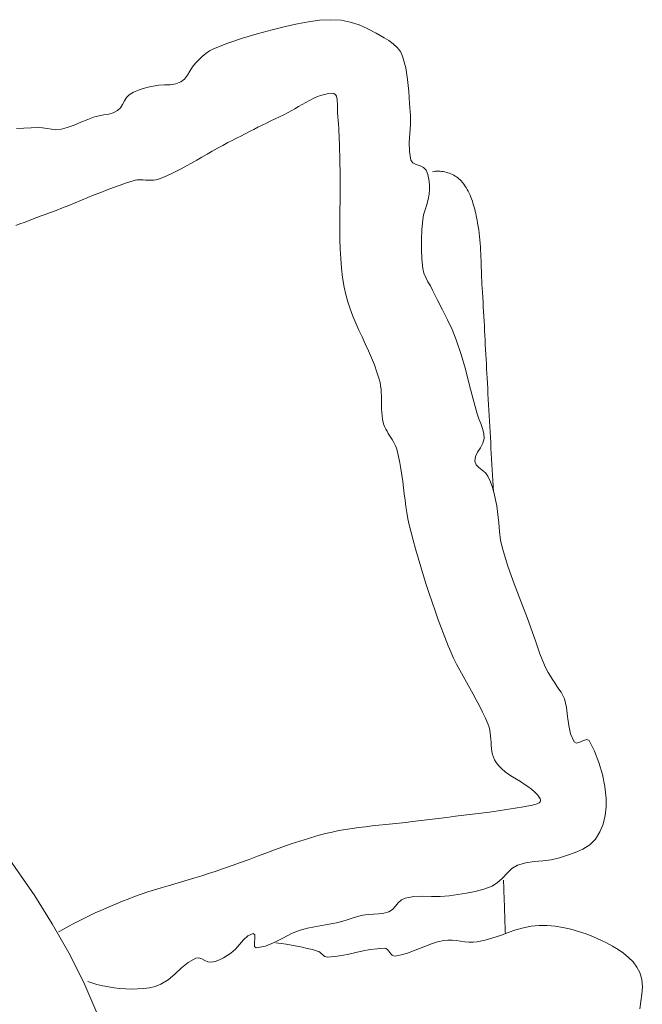
# Model space of a CAD drawing. Units: inches. Extents: x -36302355 to 648, y -221479757 to 75.
# Tile 20 of 37: x 572 to 589, y -501 to -475. Entities that reach past the tile are written whole.
import ezdxf

# ---------------------------------------------------------------- set-up
doc = ezdxf.new("R2010")
doc.units = ezdxf.units.IN
doc.header["$MEASUREMENT"] = 0
doc.layers.add('A-FURN', color=8, linetype='Continuous', lineweight=13)

# ---------------------------------------------------------------- blocks, each defined once
blk = doc.blocks.new('BED-DOUBLE')
for p, q in [((26.757, 79.348), (26.607, 79.27)), ((26.943, 79.401), (26.757, 79.348)), ((27.135, 79.418), (26.943, 79.401)), ((27.332, 79.407), (27.135, 79.418)), ((27.532, 79.381), (27.332, 79.407)), ((27.733, 79.348), (27.532, 79.381)), ((26.347, 79.049), (26.235, 78.914)), ((26.471, 79.169), (26.347, 79.049)), ((26.607, 79.27), (26.471, 79.169)), ((26.235, 78.914), (26.134, 78.768)), ((26.042, 78.615), (25.959, 78.459)), ((26.134, 78.768), (26.042, 78.615)), ((20.815, 78.133), (21.12, 78.252)), ((21.12, 78.252), (21.435, 78.344)), ((21.435, 78.344), (21.756, 78.407)), ((21.756, 78.407), (22.08, 78.443)), ((22.08, 78.443), (22.309, 78.445)), ((22.309, 78.445), (22.541, 78.42)), ((22.541, 78.42), (22.768, 78.366)), ((22.768, 78.366), (22.981, 78.28)), ((22.981, 78.28), (23.172, 78.159)), ((25.883, 78.303), (25.797, 78.108)), ((25.959, 78.459), (25.883, 78.303)), ((20.495, 77.926), (20.524, 77.986)), ((20.524, 77.986), (20.815, 78.133)), ((23.172, 78.159), (23.323, 78.006)), ((23.323, 78.006), (23.44, 77.822)), ((25.797, 78.108), (25.719, 77.908)), ((20.521, 77.836), (20.495, 77.926)), ((20.567, 77.736), (20.521, 77.836)), ((20.594, 77.646), (20.567, 77.736)), ((23.44, 77.822), (23.532, 77.618)), ((25.719, 77.908), (25.65, 77.704)), ((20.119, 77.44), (20.35, 77.491)), ((20.35, 77.491), (20.565, 77.584)), ((20.565, 77.584), (20.594, 77.646)), ((23.532, 77.618), (23.607, 77.405)), ((25.593, 77.496), (25.546, 77.286)), ((25.65, 77.704), (25.593, 77.496)), ((19.147, 77.177), (19.23, 77.234)), ((19.23, 77.234), (19.317, 77.284)), ((19.317, 77.284), (19.408, 77.323)), ((19.408, 77.323), (19.64, 77.378)), ((19.64, 77.378), (19.88, 77.41)), ((19.88, 77.41), (20.119, 77.44)), ((23.607, 77.405), (23.677, 77.194)), ((23.677, 77.194), (23.73, 76.972)), ((25.546, 77.286), (25.513, 77.074)), ((18.7, 76.891), (18.794, 76.949)), ((18.794, 76.949), (18.887, 77.007)), ((18.887, 77.007), (18.98, 77.065)), ((18.98, 77.065), (19.065, 77.119)), ((19.065, 77.119), (19.147, 77.177)), ((23.73, 76.972), (23.756, 76.743)), ((25.513, 77.074), (25.494, 76.862)), ((18.038, 76.614), (18.196, 76.668)), ((18.196, 76.668), (18.352, 76.726)), ((18.352, 76.726), (18.506, 76.789)), ((18.506, 76.789), (18.605, 76.837)), ((18.605, 76.837), (18.7, 76.891)), ((21.997, 76.607), (22.092, 76.675)), ((22.092, 76.675), (22.122, 76.687)), ((22.122, 76.687), (22.15, 76.685)), ((22.15, 76.685), (22.174, 76.67)), ((22.174, 76.67), (22.196, 76.645)), ((23.756, 76.743), (23.776, 76.512)), ((25.494, 76.862), (25.489, 76.649)), ((17.253, 76.332), (17.722, 76.507)), ((17.722, 76.507), (17.88, 76.561)), ((17.88, 76.561), (18.038, 76.614)), ((21.761, 76.345), (21.833, 76.44)), ((21.833, 76.44), (21.911, 76.527)), ((21.911, 76.527), (21.997, 76.607)), ((22.196, 76.645), (22.215, 76.61)), ((22.215, 76.61), (22.232, 76.569)), ((22.232, 76.569), (22.247, 76.522)), ((22.247, 76.522), (22.26, 76.472)), ((22.26, 76.472), (22.271, 76.419)), ((22.271, 76.419), (22.281, 76.367)), ((23.776, 76.512), (23.809, 76.285)), ((25.489, 76.649), (25.507, 76.436)), ((25.507, 76.436), (25.55, 76.227)), ((16.318, 75.975), (16.786, 76.152)), ((16.786, 76.152), (17.253, 76.332)), ((21.565, 76.038), (21.628, 76.142)), ((21.628, 76.142), (21.693, 76.245)), ((21.693, 76.245), (21.761, 76.345)), ((22.281, 76.367), (22.29, 76.317)), ((22.29, 76.317), (22.297, 76.271)), ((22.297, 76.271), (22.304, 76.23)), ((22.304, 76.23), (22.343, 76.002)), ((23.809, 76.285), (23.875, 76.067)), ((25.55, 76.227), (25.61, 76.02)), ((15.847, 75.807), (16.318, 75.975)), ((21.434, 75.833), (21.5, 75.934)), ((21.5, 75.934), (21.565, 76.038)), ((22.343, 76.002), (22.38, 75.774)), ((23.875, 76.067), (23.965, 75.917)), ((23.965, 75.917), (24.086, 75.786)), ((25.61, 76.02), (25.681, 75.814)), ((14.916, 75.581), (15.145, 75.609)), ((15.145, 75.609), (15.37, 75.658)), ((15.37, 75.658), (15.847, 75.807)), ((21.205, 75.561), (21.288, 75.644)), ((21.288, 75.644), (21.364, 75.736)), ((21.364, 75.736), (21.434, 75.833)), ((22.38, 75.774), (22.414, 75.545)), ((24.086, 75.786), (24.218, 75.662)), ((24.218, 75.662), (24.341, 75.531)), ((24.272, 75.689), (24.344, 75.691)), ((24.344, 75.691), (24.416, 75.694)), ((24.416, 75.694), (24.488, 75.697)), ((24.488, 75.697), (24.56, 75.699)), ((24.56, 75.699), (24.632, 75.702)), ((24.632, 75.702), (24.704, 75.704)), ((24.704, 75.704), (24.776, 75.707)), ((24.776, 75.707), (24.848, 75.709)), ((24.848, 75.709), (24.92, 75.712)), ((24.92, 75.712), (24.992, 75.714)), ((24.992, 75.714), (25.064, 75.717)), ((25.064, 75.717), (25.136, 75.719)), ((25.136, 75.719), (25.208, 75.722)), ((25.208, 75.722), (25.28, 75.724)), ((25.28, 75.724), (25.353, 75.727)), ((25.353, 75.727), (25.425, 75.729)), ((25.425, 75.729), (25.497, 75.732)), ((25.497, 75.732), (25.569, 75.734)), ((25.569, 75.734), (25.641, 75.737)), ((25.641, 75.737), (25.713, 75.74)), ((25.681, 75.814), (25.756, 75.609)), ((25.756, 75.609), (25.827, 75.404)), ((12.238, 75.329), (12.384, 75.337)), ((12.384, 75.337), (12.53, 75.345)), ((12.53, 75.345), (12.675, 75.353)), ((12.675, 75.353), (12.821, 75.362)), ((12.821, 75.362), (12.966, 75.37)), ((12.966, 75.37), (13.112, 75.378)), ((13.112, 75.378), (13.258, 75.386)), ((13.258, 75.386), (13.403, 75.395)), ((13.403, 75.395), (13.549, 75.403)), ((13.425, 75.27), (13.578, 75.336)), ((13.549, 75.403), (13.694, 75.411)), ((13.578, 75.336), (13.736, 75.39)), ((13.694, 75.411), (13.84, 75.419)), ((13.736, 75.39), (13.898, 75.435)), ((13.898, 75.435), (14.062, 75.473)), ((14.062, 75.473), (14.226, 75.506)), ((14.226, 75.506), (14.454, 75.541)), ((14.454, 75.541), (14.685, 75.562)), ((14.685, 75.562), (14.916, 75.581)), ((20.248, 75.322), (20.328, 75.335)), ((20.328, 75.335), (20.41, 75.344)), ((20.41, 75.344), (20.493, 75.35)), ((20.493, 75.35), (20.576, 75.355)), ((20.576, 75.355), (20.658, 75.36)), ((20.658, 75.36), (20.74, 75.367)), ((20.74, 75.367), (20.82, 75.378)), ((20.82, 75.378), (20.898, 75.394)), ((20.898, 75.394), (20.973, 75.417)), ((20.973, 75.417), (21.045, 75.447)), ((21.045, 75.447), (21.112, 75.488)), ((21.112, 75.488), (21.205, 75.561)), ((22.414, 75.545), (22.446, 75.315)), ((24.341, 75.531), (24.434, 75.383)), ((24.434, 75.383), (24.518, 75.161)), ((25.827, 75.404), (25.889, 75.196)), ((7.272, 75.067), (7.363, 75.072)), ((7.363, 75.072), (7.455, 75.077)), ((7.455, 75.077), (7.547, 75.081)), ((7.547, 75.081), (7.639, 75.085)), ((7.639, 75.085), (7.73, 75.088)), ((7.73, 75.088), (7.822, 75.091)), ((7.822, 75.091), (7.914, 75.095)), ((7.914, 75.095), (8.006, 75.098)), ((8.006, 75.098), (8.098, 75.102)), ((8.098, 75.102), (8.189, 75.106)), ((8.189, 75.106), (8.281, 75.11)), ((8.281, 75.11), (8.372, 75.116)), ((8.372, 75.116), (8.5, 75.124)), ((8.5, 75.124), (8.628, 75.131)), ((8.628, 75.131), (8.756, 75.139)), ((8.756, 75.139), (8.883, 75.146)), ((8.883, 75.146), (9.011, 75.154)), ((9.011, 75.154), (9.139, 75.161)), ((9.139, 75.161), (9.267, 75.168)), ((9.267, 75.168), (9.394, 75.175)), ((9.394, 75.175), (9.522, 75.181)), ((9.522, 75.181), (9.65, 75.188)), ((9.65, 75.188), (9.778, 75.195)), ((9.778, 75.195), (9.906, 75.201)), ((9.906, 75.201), (10.033, 75.208)), ((10.033, 75.208), (10.161, 75.215)), ((10.161, 75.215), (10.289, 75.221)), ((10.289, 75.221), (10.417, 75.228)), ((10.417, 75.228), (10.545, 75.235)), ((10.545, 75.235), (10.672, 75.242)), ((10.672, 75.242), (10.8, 75.248)), ((10.8, 75.248), (10.928, 75.255)), ((10.928, 75.255), (11.074, 75.264)), ((11.074, 75.264), (11.219, 75.272)), ((11.219, 75.272), (11.365, 75.28)), ((11.365, 75.28), (11.511, 75.288)), ((11.511, 75.288), (11.656, 75.296)), ((11.656, 75.296), (11.802, 75.304)), ((11.802, 75.304), (11.947, 75.312)), ((11.888, 75.025), (12.019, 75.077)), ((11.947, 75.312), (12.093, 75.321)), ((12.019, 75.077), (12.151, 75.125)), ((12.093, 75.321), (12.238, 75.329)), ((12.151, 75.125), (12.284, 75.159)), ((12.284, 75.159), (12.419, 75.168)), ((12.419, 75.168), (12.546, 75.136)), ((12.546, 75.136), (12.666, 75.069)), ((12.666, 75.069), (12.784, 74.994)), ((13.199, 75.028), (13.268, 75.118)), ((13.268, 75.118), (13.34, 75.205)), ((13.34, 75.205), (13.425, 75.27)), ((19.599, 75.045), (19.762, 75.127)), ((19.762, 75.127), (19.927, 75.205)), ((19.927, 75.205), (20.094, 75.277)), ((20.094, 75.277), (20.17, 75.303)), ((20.17, 75.303), (20.248, 75.322)), ((22.446, 75.315), (22.476, 75.086)), ((22.476, 75.086), (22.505, 74.856)), ((24.518, 75.161), (24.58, 74.932)), ((25.889, 75.196), (25.933, 74.985)), ((5.882, 74.79), (5.935, 74.812)), ((5.935, 74.812), (5.988, 74.832)), ((5.988, 74.832), (6.043, 74.852)), ((6.043, 74.852), (6.098, 74.869)), ((6.098, 74.869), (6.153, 74.886)), ((6.153, 74.886), (6.209, 74.902)), ((6.209, 74.902), (6.265, 74.916)), ((6.265, 74.916), (6.322, 74.93)), ((6.322, 74.93), (6.378, 74.943)), ((6.378, 74.943), (6.434, 74.955)), ((6.434, 74.955), (6.49, 74.967)), ((6.49, 74.967), (6.546, 74.978)), ((6.546, 74.978), (6.636, 74.995)), ((6.636, 74.995), (6.726, 75.01)), ((6.726, 75.01), (6.816, 75.023)), ((6.816, 75.023), (6.907, 75.034)), ((6.907, 75.034), (6.998, 75.044)), ((6.998, 75.044), (7.089, 75.053)), ((7.089, 75.053), (7.18, 75.06)), ((7.18, 75.06), (7.272, 75.067)), ((10.958, 74.77), (11.358, 74.873)), ((11.358, 74.873), (11.757, 74.981)), ((11.757, 74.981), (11.888, 75.025)), ((12.784, 74.994), (12.904, 74.935)), ((12.904, 74.935), (13.03, 74.919)), ((13.03, 74.919), (13.123, 74.955)), ((13.123, 74.955), (13.199, 75.028)), ((19.118, 74.782), (19.277, 74.871)), ((19.277, 74.871), (19.437, 74.959)), ((19.437, 74.959), (19.599, 75.045)), ((22.505, 74.856), (22.533, 74.626)), ((24.58, 74.932), (24.626, 74.698)), ((25.933, 74.985), (25.942, 74.873)), ((25.942, 74.873), (25.939, 74.761)), ((5.472, 74.521), (5.501, 74.549)), ((5.501, 74.549), (5.544, 74.587)), ((5.544, 74.587), (5.588, 74.622)), ((5.588, 74.622), (5.633, 74.654)), ((5.633, 74.654), (5.68, 74.685)), ((5.68, 74.685), (5.729, 74.714)), ((5.729, 74.714), (5.779, 74.741)), ((5.779, 74.741), (5.83, 74.766)), ((5.83, 74.766), (5.882, 74.79)), ((9.77, 74.421), (10.161, 74.551)), ((10.161, 74.551), (10.558, 74.665)), ((10.558, 74.665), (10.958, 74.77)), ((18.638, 74.516), (18.798, 74.603)), ((18.798, 74.603), (18.958, 74.692)), ((18.958, 74.692), (19.118, 74.782)), ((22.533, 74.626), (22.56, 74.396)), ((24.626, 74.698), (24.663, 74.462)), ((25.927, 74.648), (25.911, 74.534)), ((25.939, 74.761), (25.927, 74.648)), ((5.299, 74.237), (5.314, 74.277)), ((5.314, 74.277), (5.332, 74.316)), ((5.332, 74.316), (5.351, 74.353)), ((5.351, 74.353), (5.372, 74.39)), ((5.372, 74.39), (5.395, 74.425)), ((5.395, 74.425), (5.419, 74.459)), ((5.419, 74.459), (5.445, 74.491)), ((5.445, 74.491), (5.472, 74.521)), ((9.228, 74.184), (9.496, 74.31)), ((9.496, 74.31), (9.77, 74.421)), ((18.148, 74.273), (18.313, 74.35)), ((18.313, 74.35), (18.476, 74.431)), ((18.476, 74.431), (18.638, 74.516)), ((22.56, 74.396), (22.588, 74.166)), ((24.663, 74.462), (24.695, 74.226)), ((25.884, 74.308), (25.882, 74.196)), ((25.895, 74.421), (25.884, 74.308)), ((25.911, 74.534), (25.895, 74.421)), ((5.244, 73.988), (5.248, 74.03)), ((5.248, 74.03), (5.254, 74.072)), ((5.254, 74.072), (5.262, 74.114)), ((5.262, 74.114), (5.273, 74.156)), ((5.273, 74.156), (5.285, 74.197)), ((5.285, 74.197), (5.299, 74.237)), ((8.701, 73.914), (8.965, 74.05)), ((8.965, 74.05), (9.228, 74.184)), ((17.282, 73.935), (17.515, 74.022)), ((17.515, 74.022), (17.748, 74.11)), ((17.748, 74.11), (17.98, 74.202)), ((17.98, 74.202), (18.148, 74.273)), ((22.588, 74.166), (22.615, 73.936)), ((24.695, 74.226), (24.712, 73.99)), ((25.882, 74.196), (25.893, 74.084)), ((25.893, 74.084), (25.931, 73.917)), ((5.242, 73.946), (5.244, 73.988)), ((5.242, 73.905), (5.242, 73.946)), ((5.245, 73.864), (5.242, 73.905)), ((5.249, 73.823), (5.245, 73.864)), ((5.256, 73.784), (5.249, 73.823)), ((8.321, 73.724), (8.436, 73.783)), ((8.436, 73.783), (8.701, 73.914)), ((16.575, 73.69), (16.812, 73.769)), ((16.812, 73.769), (17.047, 73.851)), ((17.047, 73.851), (17.282, 73.935)), ((22.615, 73.936), (22.643, 73.706)), ((24.71, 73.753), (24.706, 73.515)), ((24.712, 73.99), (24.71, 73.753)), ((25.931, 73.917), (25.983, 73.753)), ((25.983, 73.753), (26.044, 73.592)), ((5.102, 73.448), (5.146, 73.544)), ((5.146, 73.544), (5.214, 73.612)), ((5.214, 73.612), (5.335, 73.661)), ((5.335, 73.661), (5.463, 73.688)), ((5.463, 73.688), (5.596, 73.698)), ((5.596, 73.698), (5.731, 73.697)), ((5.731, 73.697), (5.863, 73.69)), ((5.863, 73.69), (6.003, 73.668)), ((6.003, 73.668), (6.139, 73.629)), ((6.139, 73.629), (6.275, 73.584)), ((6.275, 73.584), (6.411, 73.544)), ((6.411, 73.544), (6.55, 73.52)), ((6.55, 73.52), (6.81, 73.5)), ((6.81, 73.5), (7.072, 73.487)), ((7.072, 73.487), (7.333, 73.484)), ((7.333, 73.484), (7.594, 73.494)), ((7.594, 73.494), (7.853, 73.521)), ((7.853, 73.521), (7.976, 73.551)), ((7.976, 73.551), (8.094, 73.6)), ((8.094, 73.6), (8.208, 73.66)), ((8.208, 73.66), (8.321, 73.724)), ((15.862, 73.465), (16.101, 73.538)), ((16.101, 73.538), (16.338, 73.612)), ((16.338, 73.612), (16.575, 73.69)), ((22.643, 73.706), (22.672, 73.476)), ((24.706, 73.515), (24.715, 73.279)), ((26.044, 73.592), (26.109, 73.431)), ((4.945, 73.202), (5.019, 73.255)), ((5.019, 73.255), (5.066, 73.344)), ((5.066, 73.344), (5.102, 73.448)), ((14.902, 73.196), (15.143, 73.26)), ((15.143, 73.26), (15.383, 73.326)), ((15.383, 73.326), (15.623, 73.395)), ((15.623, 73.395), (15.862, 73.465)), ((22.672, 73.476), (22.703, 73.247)), ((22.703, 73.247), (22.726, 73.067)), ((24.715, 73.279), (24.755, 73.049)), ((26.109, 73.431), (26.174, 73.271)), ((26.174, 73.271), (26.233, 73.109)), ((2.033, 72.919), (2.158, 72.979)), ((2.158, 72.979), (2.468, 73.062)), ((2.468, 73.062), (2.784, 73.114)), ((2.784, 73.114), (3.106, 73.145)), ((3.106, 73.145), (3.429, 73.167)), ((3.429, 73.167), (3.751, 73.188)), ((3.751, 73.188), (3.991, 73.191)), ((3.991, 73.191), (4.232, 73.175)), ((4.232, 73.175), (4.474, 73.159)), ((4.474, 73.159), (4.712, 73.161)), ((4.712, 73.161), (4.945, 73.202)), ((13.235, 72.933), (13.402, 72.958)), ((13.402, 72.958), (13.57, 72.981)), ((13.57, 72.981), (13.738, 73.003)), ((13.738, 73.003), (13.905, 73.023)), ((13.905, 73.023), (14.073, 73.045)), ((14.073, 73.045), (14.24, 73.068)), ((14.24, 73.068), (14.407, 73.094)), ((14.407, 73.094), (14.573, 73.123)), ((14.573, 73.123), (14.738, 73.157)), ((14.738, 73.157), (14.902, 73.196)), ((22.726, 73.067), (22.746, 72.887)), ((24.755, 73.049), (24.805, 72.949)), ((26.233, 73.109), (26.28, 72.944)), ((1.735, 72.608), (1.822, 72.725)), ((1.822, 72.725), (1.921, 72.832)), ((1.921, 72.832), (2.033, 72.919)), ((12.392, 72.663), (12.448, 72.698)), ((12.448, 72.698), (12.504, 72.732)), ((12.504, 72.732), (12.56, 72.763)), ((12.56, 72.763), (12.619, 72.791)), ((12.619, 72.791), (12.678, 72.815)), ((12.678, 72.815), (12.74, 72.833)), ((12.74, 72.833), (12.904, 72.872)), ((12.904, 72.872), (13.069, 72.905)), ((13.069, 72.905), (13.235, 72.933)), ((22.746, 72.887), (22.765, 72.706)), ((22.765, 72.706), (22.784, 72.525)), ((24.805, 72.949), (24.884, 72.864)), ((24.884, 72.864), (24.976, 72.786)), ((24.976, 72.786), (25.061, 72.704)), ((25.061, 72.704), (25.122, 72.608)), ((26.286, 72.699), (26.252, 72.666)), ((26.28, 72.944), (26.312, 72.776)), ((26.308, 72.735), (26.286, 72.699)), ((26.312, 72.776), (26.308, 72.735)), ((1.534, 72.267), (1.658, 72.486)), ((1.658, 72.486), (1.735, 72.608)), ((11.723, 72.419), (11.813, 72.427)), ((11.813, 72.427), (11.901, 72.44)), ((11.901, 72.44), (11.989, 72.458)), ((11.989, 72.458), (12.05, 72.477)), ((12.05, 72.477), (12.11, 72.501)), ((12.11, 72.501), (12.168, 72.529)), ((12.168, 72.529), (12.225, 72.56)), ((12.225, 72.56), (12.281, 72.593)), ((12.281, 72.593), (12.337, 72.628)), ((12.337, 72.628), (12.392, 72.663)), ((22.784, 72.525), (22.802, 72.344)), ((25.122, 72.608), (25.161, 72.474)), ((25.161, 72.474), (25.18, 72.335)), ((26.111, 72.533), (26.102, 72.492)), ((26.102, 72.492), (26.114, 72.299)), ((26.136, 72.57), (26.111, 72.533)), ((26.172, 72.603), (26.136, 72.57)), ((26.212, 72.634), (26.172, 72.603)), ((26.252, 72.666), (26.212, 72.634)), ((1.417, 72.042), (1.534, 72.267)), ((10.253, 72.144), (10.442, 72.221)), ((10.442, 72.221), (10.634, 72.291)), ((10.634, 72.291), (10.828, 72.353)), ((10.828, 72.353), (10.915, 72.374)), ((10.915, 72.374), (11.003, 72.389)), ((11.003, 72.389), (11.092, 72.399)), ((11.092, 72.399), (11.181, 72.406)), ((11.181, 72.406), (11.271, 72.409)), ((11.271, 72.409), (11.362, 72.41)), ((11.362, 72.41), (11.453, 72.411)), ((11.453, 72.411), (11.543, 72.412)), ((11.543, 72.412), (11.634, 72.414)), ((11.634, 72.414), (11.723, 72.419)), ((22.802, 72.344), (22.82, 72.164)), ((22.82, 72.164), (22.84, 71.983)), ((25.18, 72.335), (25.188, 72.193)), ((25.188, 72.193), (25.197, 72.051)), ((26.114, 72.299), (26.14, 72.108)), ((1.316, 71.81), (1.417, 72.042)), ((9.692, 71.891), (9.878, 71.977)), ((9.878, 71.977), (10.065, 72.062)), ((10.065, 72.062), (10.253, 72.144)), ((22.84, 71.983), (22.862, 71.803)), ((25.197, 72.051), (25.217, 71.912)), ((25.217, 71.912), (25.252, 71.769)), ((26.14, 72.108), (26.176, 71.917)), ((26.176, 71.917), (26.217, 71.727)), ((1.238, 71.572), (1.316, 71.81)), ((8.94, 71.57), (9.13, 71.643)), ((9.13, 71.643), (9.318, 71.722)), ((9.318, 71.722), (9.506, 71.805)), ((9.506, 71.805), (9.692, 71.891)), ((22.862, 71.803), (22.886, 71.623)), ((25.252, 71.769), (25.294, 71.628)), ((26.217, 71.727), (26.258, 71.537)), ((1.19, 71.327), (1.238, 71.572)), ((7.845, 71.338), (8.1, 71.368)), ((8.1, 71.368), (8.354, 71.408)), ((8.354, 71.408), (8.553, 71.451)), ((8.553, 71.451), (8.748, 71.506)), ((8.748, 71.506), (8.94, 71.57)), ((22.886, 71.623), (22.914, 71.444)), ((22.914, 71.444), (22.945, 71.266)), ((25.294, 71.628), (25.339, 71.487)), ((25.339, 71.487), (25.382, 71.346)), ((26.258, 71.537), (26.296, 71.346)), ((1.175, 71.036), (1.19, 71.327)), ((3.15, 71.095), (3.155, 71.133)), ((3.155, 71.133), (3.171, 71.163)), ((3.171, 71.163), (3.197, 71.186)), ((3.197, 71.186), (3.231, 71.202)), ((3.231, 71.202), (3.271, 71.214)), ((3.271, 71.214), (3.318, 71.222)), ((3.318, 71.222), (3.368, 71.226)), ((3.368, 71.226), (3.421, 71.228)), ((3.421, 71.228), (3.475, 71.228)), ((3.475, 71.228), (3.529, 71.228)), ((3.529, 71.228), (3.581, 71.228)), ((3.581, 71.228), (3.63, 71.229)), ((3.63, 71.229), (3.674, 71.232)), ((3.674, 71.232), (3.776, 71.243)), ((3.776, 71.243), (3.879, 71.251)), ((3.879, 71.251), (3.981, 71.258)), ((3.981, 71.258), (4.083, 71.264)), ((4.083, 71.264), (4.186, 71.27)), ((4.186, 71.27), (4.288, 71.274)), ((4.288, 71.274), (4.391, 71.277)), ((4.391, 71.277), (4.494, 71.281)), ((4.494, 71.281), (4.596, 71.283)), ((4.596, 71.283), (4.699, 71.286)), ((4.699, 71.286), (4.801, 71.289)), ((4.801, 71.289), (4.904, 71.292)), ((4.904, 71.292), (5.007, 71.296)), ((5.007, 71.296), (5.264, 71.303)), ((5.264, 71.303), (5.523, 71.305)), ((5.523, 71.305), (5.781, 71.304)), ((5.781, 71.304), (6.04, 71.301)), ((6.04, 71.301), (6.299, 71.297)), ((6.299, 71.297), (6.558, 71.294)), ((6.558, 71.294), (6.816, 71.293)), ((6.816, 71.293), (7.074, 71.296)), ((7.074, 71.296), (7.332, 71.303)), ((7.332, 71.303), (7.589, 71.317)), ((7.589, 71.317), (7.845, 71.338)), ((22.945, 71.266), (22.982, 71.089)), ((25.382, 71.346), (25.42, 71.204)), ((25.42, 71.204), (25.46, 71.009)), ((26.296, 71.346), (26.325, 71.155)), ((26.325, 71.155), (26.341, 70.962)), ((1.191, 70.743), (1.175, 71.036)), ((3.16, 70.987), (3.15, 71.095)), ((3.18, 70.881), (3.16, 70.987)), ((3.21, 70.777), (3.18, 70.881)), ((22.982, 71.089), (23.023, 70.912)), ((23.023, 70.912), (23.085, 70.679)), ((25.46, 71.009), (25.493, 70.813)), ((26.298, 70.858), (26.271, 70.827)), ((26.321, 70.891), (26.298, 70.858)), ((26.336, 70.925), (26.321, 70.891)), ((26.341, 70.962), (26.336, 70.925)), ((1.231, 70.451), (1.191, 70.743)), ((3.248, 70.675), (3.21, 70.777)), ((3.292, 70.575), (3.248, 70.675)), ((3.341, 70.476), (3.292, 70.575)), ((23.085, 70.679), (23.153, 70.448)), ((25.493, 70.813), (25.525, 70.617)), ((25.525, 70.617), (25.564, 70.423)), ((26.177, 70.695), (26.14, 70.556)), ((26.192, 70.731), (26.177, 70.695)), ((26.215, 70.764), (26.192, 70.731)), ((26.242, 70.796), (26.215, 70.764)), ((26.271, 70.827), (26.242, 70.796)), ((1.287, 70.16), (1.231, 70.451)), ((3.395, 70.377), (3.341, 70.476)), ((3.451, 70.28), (3.395, 70.377)), ((23.153, 70.448), (23.225, 70.218)), ((25.564, 70.423), (25.614, 70.231)), ((26.106, 70.417), (26.074, 70.278)), ((26.14, 70.556), (26.106, 70.417)), ((1.35, 69.873), (1.287, 70.16)), ((3.509, 70.182), (3.451, 70.28)), ((3.566, 70.085), (3.509, 70.182)), ((3.622, 69.988), (3.566, 70.085)), ((23.225, 70.218), (23.302, 69.989)), ((25.614, 70.231), (25.71, 69.993)), ((26.045, 70.138), (26.019, 69.997)), ((26.074, 70.278), (26.045, 70.138)), ((1.446, 69.472), (1.35, 69.873)), ((3.676, 69.89), (3.622, 69.988)), ((3.725, 69.791), (3.676, 69.89)), ((3.78, 69.675), (3.725, 69.791)), ((23.302, 69.989), (23.381, 69.761)), ((25.71, 69.993), (25.829, 69.762)), ((25.995, 69.856), (25.974, 69.714)), ((26.019, 69.997), (25.995, 69.856)), ((3.836, 69.558), (3.78, 69.675)), ((3.893, 69.442), (3.836, 69.558)), ((23.381, 69.761), (23.463, 69.534)), ((23.463, 69.534), (23.547, 69.307)), ((25.829, 69.762), (25.948, 69.531)), ((25.948, 69.531), (26.043, 69.295)), ((25.974, 69.714), (25.956, 69.572)), ((1.554, 69.073), (1.446, 69.472)), ((3.949, 69.326), (3.893, 69.442)), ((4.007, 69.21), (3.949, 69.326)), ((23.547, 69.307), (23.632, 69.08)), ((26.043, 69.295), (26.093, 69.048)), ((1.675, 68.678), (1.554, 69.073)), ((4.064, 69.095), (4.007, 69.21)), ((4.122, 68.979), (4.064, 69.095)), ((23.632, 69.08), (23.716, 68.854)), ((25.738, 69.008), (25.707, 68.962)), ((25.834, 69.01), (25.738, 69.008)), ((25.954, 68.998), (25.834, 69.01)), ((26.054, 69.001), (25.954, 68.998)), ((26.093, 69.048), (26.054, 69.001)), ((4.18, 68.864), (4.122, 68.979)), ((4.239, 68.749), (4.18, 68.864)), ((4.298, 68.634), (4.239, 68.749)), ((23.716, 68.854), (23.801, 68.627)), ((25.707, 68.962), (25.768, 68.822)), ((25.768, 68.822), (25.873, 68.704)), ((1.809, 68.288), (1.675, 68.678)), ((4.357, 68.519), (4.298, 68.634)), ((4.416, 68.404), (4.357, 68.519)), ((23.801, 68.627), (23.883, 68.4)), ((25.873, 68.704), (25.999, 68.598)), ((25.999, 68.598), (26.127, 68.49)), ((26.127, 68.49), (26.234, 68.369)), ((1.956, 67.902), (1.809, 68.288)), ((4.475, 68.289), (4.416, 68.404)), ((4.55, 68.148), (4.475, 68.289)), ((23.883, 68.4), (23.964, 68.172)), ((26.234, 68.369), (26.299, 68.27)), ((26.299, 68.27), (26.36, 68.166)), ((4.627, 68.007), (4.55, 68.148)), ((4.705, 67.868), (4.627, 68.007)), ((23.964, 68.172), (24.041, 67.944)), ((24.041, 67.944), (24.1, 67.764)), ((26.36, 68.166), (26.413, 68.059)), ((26.413, 68.059), (26.454, 67.948)), ((26.454, 67.948), (26.479, 67.833)), ((2.012, 67.792), (1.956, 67.902)), ((2.082, 67.69), (2.012, 67.792)), ((2.164, 67.594), (2.082, 67.69)), ((4.785, 67.729), (4.705, 67.868)), ((4.865, 67.59), (4.785, 67.729)), ((24.1, 67.764), (24.156, 67.584)), ((26.469, 67.749), (26.431, 67.667)), ((26.479, 67.833), (26.469, 67.749)), ((2.251, 67.503), (2.164, 67.594)), ((2.34, 67.415), (2.251, 67.503)), ((2.441, 67.335), (2.34, 67.415)), ((4.945, 67.451), (4.865, 67.59)), ((5.025, 67.311), (4.945, 67.451)), ((24.156, 67.584), (24.211, 67.403)), ((24.211, 67.403), (24.264, 67.222)), ((26.386, 67.585), (26.357, 67.505)), ((26.357, 67.505), (26.365, 67.427)), ((26.365, 67.427), (26.483, 67.224)), ((26.431, 67.667), (26.386, 67.585)), ((2.555, 67.267), (2.441, 67.335)), ((2.668, 67.2), (2.555, 67.267)), ((2.769, 67.123), (2.668, 67.2)), ((5.102, 67.171), (5.025, 67.311)), ((5.178, 67.03), (5.102, 67.171)), ((24.264, 67.222), (24.318, 67.041)), ((26.483, 67.224), (26.632, 67.041)), ((2.846, 67.024), (2.769, 67.123)), ((2.898, 66.886), (2.846, 67.024)), ((2.92, 66.738), (2.898, 66.886)), ((5.252, 66.888), (5.178, 67.03)), ((5.322, 66.745), (5.252, 66.888)), ((24.318, 67.041), (24.371, 66.86)), ((26.632, 67.041), (26.794, 66.864)), ((2.927, 66.585), (2.92, 66.738)), ((5.388, 66.599), (5.322, 66.745)), ((24.371, 66.86), (24.424, 66.679)), ((24.424, 66.679), (24.479, 66.498)), ((26.794, 66.864), (26.947, 66.682)), ((26.947, 66.682), (27.07, 66.482)), ((2.934, 66.432), (2.927, 66.585)), ((2.957, 66.283), (2.934, 66.432)), ((5.45, 66.452), (5.388, 66.599)), ((5.467, 66.4), (5.45, 66.452)), ((5.478, 66.347), (5.467, 66.4)), ((5.485, 66.293), (5.478, 66.347)), ((24.479, 66.498), (24.534, 66.317)), ((27.07, 66.482), (27.127, 66.334)), ((2.99, 66.148), (2.957, 66.283)), ((3.026, 66.014), (2.99, 66.148)), ((5.48, 66.07), (5.483, 66.126)), ((5.483, 66.126), (5.486, 66.183)), ((5.487, 66.238), (5.485, 66.293)), ((5.486, 66.183), (5.487, 66.238)), ((24.534, 66.317), (24.592, 66.138)), ((24.592, 66.138), (24.652, 65.959)), ((27.127, 66.334), (27.163, 66.178)), ((27.163, 66.178), (27.184, 66.017)), ((3.068, 65.882), (3.026, 66.014)), ((3.122, 65.755), (3.068, 65.882)), ((5.474, 65.958), (5.476, 66.014)), ((5.474, 65.902), (5.474, 65.958)), ((5.478, 65.847), (5.474, 65.902)), ((5.476, 66.014), (5.48, 66.07)), ((5.486, 65.793), (5.478, 65.847)), ((24.652, 65.959), (24.715, 65.781)), ((27.184, 66.017), (27.194, 65.855)), ((27.194, 65.855), (27.198, 65.694)), ((3.19, 65.637), (3.122, 65.755)), ((3.264, 65.562), (3.19, 65.637)), ((3.356, 65.506), (3.264, 65.562)), ((5.499, 65.74), (5.486, 65.793)), ((5.555, 65.564), (5.499, 65.74)), ((5.615, 65.389), (5.555, 65.564)), ((24.715, 65.781), (24.781, 65.604)), ((24.781, 65.604), (24.839, 65.456)), ((27.198, 65.694), (27.195, 65.541)), ((3.454, 65.455), (3.356, 65.506)), ((3.545, 65.398), (3.454, 65.455)), ((3.617, 65.322), (3.545, 65.398)), ((3.672, 65.208), (3.617, 65.322)), ((5.678, 65.215), (5.615, 65.389)), ((24.839, 65.456), (24.899, 65.309)), ((24.899, 65.309), (24.96, 65.162)), ((27.182, 65.388), (27.161, 65.236)), ((27.195, 65.541), (27.182, 65.388)), ((3.707, 65.086), (3.672, 65.208)), ((3.731, 64.958), (3.707, 65.086)), ((5.744, 65.043), (5.678, 65.215)), ((5.812, 64.871), (5.744, 65.043)), ((24.96, 65.162), (25.023, 65.015)), ((27.135, 65.084), (27.108, 64.932)), ((27.161, 65.236), (27.135, 65.084)), ((3.755, 64.83), (3.731, 64.958)), ((3.787, 64.705), (3.755, 64.83)), ((5.881, 64.699), (5.812, 64.871)), ((25.023, 65.015), (25.088, 64.87)), ((25.088, 64.87), (25.154, 64.725)), ((27.839, 64.768), (27.022, 64.416)), ((27.072, 64.767), (27.05, 64.686)), ((27.092, 64.849), (27.072, 64.767)), ((27.108, 64.932), (27.092, 64.849)), ((3.854, 64.521), (3.787, 64.705)), ((3.93, 64.339), (3.854, 64.521)), ((5.951, 64.528), (5.881, 64.699)), ((6.021, 64.357), (5.951, 64.528)), ((25.154, 64.725), (25.222, 64.581)), ((25.222, 64.581), (25.292, 64.438)), ((27.023, 64.605), (26.994, 64.526)), ((27.05, 64.686), (27.023, 64.605)), ((4.005, 64.157), (3.93, 64.339)), ((6.092, 64.186), (6.021, 64.357)), ((25.292, 64.438), (25.363, 64.295)), ((25.363, 64.295), (25.436, 64.153)), ((27.022, 64.416), (26.225, 64.013)), ((4.071, 63.972), (4.005, 64.157)), ((4.119, 63.783), (4.071, 63.972)), ((6.161, 64.014), (6.092, 64.186)), ((6.229, 63.842), (6.161, 64.014)), ((25.436, 64.153), (25.511, 64.013)), ((26.225, 64.013), (25.45, 63.569)), ((25.511, 64.013), (25.586, 63.873)), ((4.128, 63.666), (4.119, 63.783)), ((6.296, 63.67), (6.229, 63.842)), ((25.586, 63.873), (25.664, 63.734)), ((4.097, 63.43), (4.117, 63.548)), ((4.117, 63.548), (4.128, 63.666)), ((6.36, 63.496), (6.296, 63.67)), ((6.401, 63.383), (6.36, 63.496)), ((25.45, 63.569), (24.695, 63.097)), ((4.072, 63.192), (4.078, 63.311)), ((4.076, 62.999), (4.072, 63.192)), ((4.078, 63.311), (4.097, 63.43)), ((6.444, 63.269), (6.401, 63.383)), ((6.488, 63.156), (6.444, 63.269)), ((4.083, 62.806), (4.076, 62.999)), ((6.531, 63.043), (6.488, 63.156)), ((6.574, 62.929), (6.531, 63.043)), ((6.616, 62.816), (6.574, 62.929)), ((24.695, 63.097), (23.379, 62.192)), ((4.096, 62.613), (4.083, 62.806)), ((6.657, 62.702), (6.616, 62.816)), ((6.696, 62.587), (6.657, 62.702))]:
    blk.add_line(p, q)

msp = doc.modelspace()

# ---------------------------------------------------------------- block references
at = {"layer": 'A-FURN', "rotation": 270}
msp.add_blockref('BED-DOUBLE', (509.53, -473.482), dxfattribs=at)

doc.saveas('drawing.dxf')
